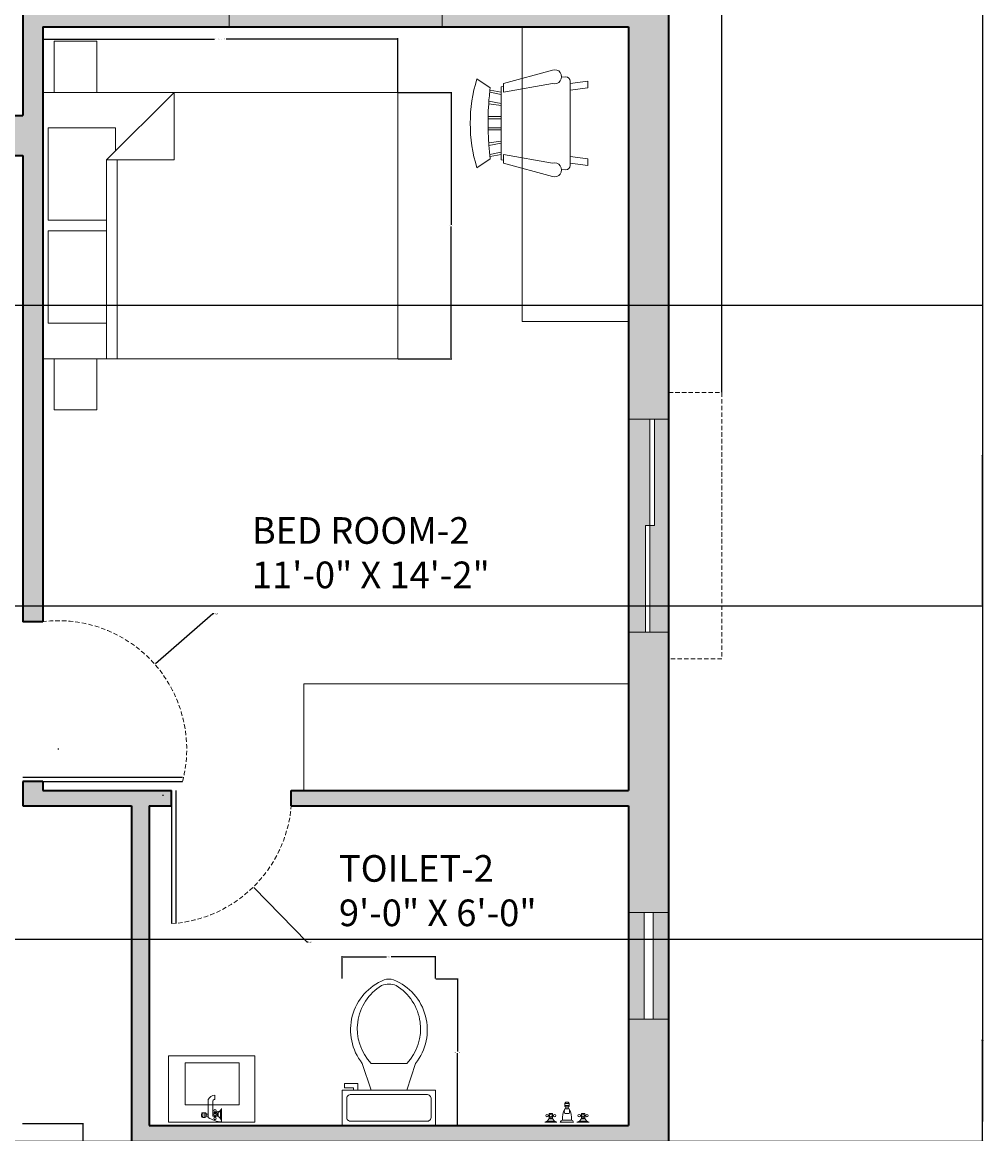
# Model space of a CAD drawing. Units: inches. Extents: x 1693 to 2974, y 2201 to 2965.
# Tile 23 of 24: x 2757 to 2973, y 2588 to 2838. Entities that reach past the tile are written whole.
import ezdxf

# ---------------------------------------------------------------- set-up
doc = ezdxf.new("R2010")
doc.units = ezdxf.units.IN
doc.header["$LTSCALE"] = 2
doc.header["$MEASUREMENT"] = 0
doc.linetypes.add('HIDDEN', pattern=[0.375, 0.25, -0.125])
for name, color, linetype, lineweight in [('A-ANNO-DIMS', 2, 'Continuous', 18), ('A-AREA-IDEN', 7, 'Continuous', 18), ('A-DOOR', 3, 'Continuous', 25), ('A-DOOR-SWNG', 3, 'HIDDEN', 13), ('A-FLOR-CASE', 32, 'Continuous', 18), ('A-FLOR-FIXT', 9, 'Continuous', 18), ('A-FURN', 8, 'Continuous', 18), ('A-GLAZ', 4, 'Continuous', 18), ('A-GLAZ-OVHD', 8, 'HIDDEN', 13), ('A-WALL', 7, 'Continuous', 35)]:
    doc.layers.add(name, color=color, linetype=linetype, lineweight=lineweight)
doc.layers.add('A-GLAZ-PATT', color=141, linetype='Continuous', lineweight=13, true_color=0xadddf7)
doc.layers.add('A-WALL-PATT', color=251, linetype='Continuous', lineweight=13, true_color=0x636466)
doc.styles.get("Standard").update_dxf_attribs({"font": 'arial.ttf'})
doc.dimstyles.get("Standard").update_dxf_attribs({"dimtxt": 0.18, "dimasz": 0.18, "dimexe": 0.18, "dimexo": 0.0625, "dimgap": 0.09, "dimtad": 0, "dimtih": 1, "dimtoh": 1, "dimdec": 1, "dimzin": 0, "dimdsep": 46, "dimlunit": 3, "dimtxsty": 'Standard', "dimcen": 0.09, "dimadec": 0, "dimazin": 0, "dimtfac": 1, "dimtdec": 1, "dimtofl": 0, "dimtmove": 0, "dimatfit": 3, "dimfxl": 1, "dimtolj": 1, "dimtzin": 0, "dimarcsym": 0})

# ---------------------------------------------------------------- blocks, each defined once
blk = doc.blocks.new('Chair - Rocking')
for p, q in [((-8, -4.5), (-10, -1.5)), ((8, -4.5), (10, -1.5)), ((-7.5, -4.5), (-7, -7)), ((-6.5, -7), (-7.02225, -4.43)), ((-4.5, -7), (-4.96674, -4.19951)), ((-4, -7), (-4.40532, -4.16272)), ((-1.5, -4.05012), (-1.5, -7)), ((-1, -7), (-1, -4.05012)), ((1, -7), (1, -4.04655)), ((1.5, -4.05012), (1.5, -7)), ((4, -7), (4.40187, -4.18694)), ((4.5, -7), (4.96761, -4.19437)), ((6.5, -7), (7, -4.4057)), ((7.5, -4.5), (7, -7)), ((-9, -7.5), (-12, -18.49999)), ((-7, -7.5), (-9, -7.5)), ((-9, -18.49999), (-7, -7.5)), ((-8.23428, -6.99939), (-8.3093, -7.47958)), ((-8.23041, -7), (8.23915, -7)), ((7, -7.5), (9, -7.5)), ((9, -18.49999), (7, -7.5)), ((8.31071, -7.48854), (8.23449, -7.00073)), ((9, -7.5), (12, -18.49999)), ((-10.36644, -20.64523), (-10.5, -21.49999)), ((-9, -22.49999), (-9.5, -26.49999)), ((0, -22.49999), (-9.5, -22.49999)), ((-8, -26.49999), (-7.5, -22.49999)), ((0, -22.49999), (9.5, -22.49999)), ((8, -26.49999), (7.5, -22.49999)), ((9, -22.49999), (9.5, -26.49999)), ((10.5, -21.49999), (10.3575, -20.58798)), ((-9.5, -26.49999), (-8, -26.49999)), ((9.5, -26.49999), (8, -26.49999))]:
    blk.add_line(p, q)
for centre, radius, start, end in [((0, -34.08333), 34.08333, 72.93847, 107.0615), ((0, -68.25004), 64.25, 93.92211, 97.15267), ((0, -68.25004), 64.25, 82.84733, 93.92211), ((-10.5, -18.99999), 1.58114, 161.5651, 18.43495), ((10.5, -18.99999), 1.58114, 161.5651, 18.43495), ((-9.5, -21.49999), 1, 180, 270), ((9.5, -21.49999), 1, 270, 0)]:
    blk.add_arc(centre, radius, start, end)
blk = doc.blocks.new('Toilet - top')
for p, q in [((9.5, -6), (9.5, -2)), ((-10, -8.5), (-8, -8.5)), ((-10, -9.5), (-10, -8.5)), ((-7, -9.5), (-10, -9.5)), ((-8, -8.5), (-8, -8)), ((-7, -8), (-7, -9.5)), ((-4, -8), (-6, -14)), ((4, -8), (6, -14)), ((4, -14), (-4, -14))]:
    blk.add_line(p, q)
blk.add_lwpolyline([(10.5, -8), (10.5, 0), (-10.5, 0), (-10.5, -8)], close=True)
for points in [[(-9.5, -2), (-9.5, -6)], [(8.5, -1), (-8.5, -1)], [(-8.5, -7), (8.5, -7)]]:
    blk.add_lwpolyline(points)
for centre, radius, start, end in [((-8.62, -1.88), 0.884, 81.8699, 188.1301), ((8.62, -1.88), 0.884, 351.8699, 98.1301), ((-8.62, -6.12), 0.884, 171.8699, 278.1301), ((8.62, -6.12), 0.884, 261.8699, 8.1301), ((3.52, -21.58), 12.17, 141.4691, 247.9714), ((4.2, -21.82), 11.33, 136.3677, 238.9468), ((-3.52, -21.58), 12.17, 292.0284, 38.5307), ((-4.2, -21.82), 11.33, 301.053, 43.6321), ((0, -27.88), 4, 245.7318, 294.2682), ((0, -29), 4, 254.8605, 285.1395)]:
    blk.add_arc(centre, radius, start, end)
blk = doc.blocks.new('Faucet - Bathroom side')
for p, q in [((-0.625, 4.25), (0.375, 4.25)), ((0.375, 3.75), (-0.625, 3.75)), ((-0.625, 3), (3.375, 3)), ((-0.375, 3), (-0.375, 3.5)), ((0.125, 3.5), (0.125, 3)), ((-1.625, 0), (-1.375, 0)), ((-1.375, 0), (1.375, 0)), ((-0.88366, 0.25), (0.88424, 0.25)), ((-0.375, 1.625), (-0.625, 1.625)), ((-0.375, 1.375), (-0.625, 1.375)), ((0.48078, 0.75), (-0.47286, 0.75)), ((2.875, 2), (0.375, 2)), ((0.375, 1.625), (0.625, 1.625)), ((0.375, 1.375), (0.625, 1.375)), ((4.375, 1.5), (3.375, 1.5))]:
    blk.add_line(p, q)
for points in [[(-0.625, 3.75), (-0.625, 4.25)], [(-0.375, 4.5), (0.125, 4.5)], [(0.125, 3.5), (-0.375, 3.5)], [(0.375, 4.25), (0.375, 3.75)]]:
    blk.add_lwpolyline(points)
blk.add_lwpolyline([(-0.375, 1), (-0.375, 2), (0.375, 2), (0.375, 1)], close=True)
for centre in [(-0.875, 1.5), (0, 1.5), (0.875, 1.5)]:
    blk.add_circle(centre, 0.27951)
for centre, radius, start, end in [((3.45929, -0.0281), 5.08436, 143.4467, 179.6834), ((-0.38253, 4.2575), 0.24259, 88.22243, 181.7776), ((-0.38253, 3.7424), 0.24259, 178.2224, 271.7776), ((0.13252, 4.2575), 0.24259, 358.2224, 91.77757), ((0.13252, 3.7424), 0.24259, 268.2224, 1.777565), ((2.70708, 1.4714), 1.66816, 0.9827695, 66.39737), ((-1.75, 1.375), 1.42522, 285.2551, 344.7449), ((1.75, 1.375), 1.42522, 195.2551, 254.7449), ((-2.49562, -0.286), 3.38273, 9.709485, 29.48735), ((2.96867, 1.5936), 0.41699, 347.0192, 102.9808)]:
    blk.add_arc(centre, radius, start, end)
blk = doc.blocks.new('Faucet - Bathroom front')
for p, q in [((-0.5, 4.25), (0.5, 4.25)), ((0.5, 3.75), (-0.5, 3.75)), ((-0.5, 3), (0.5, 3)), ((-0.25, 3), (-0.25, 3.5)), ((0.25, 3.5), (0.25, 3)), ((-5, 0), (-2.25, 0)), ((-4.5087, 0.25), (-2.7408, 0.25)), ((-4, 1.625), (-4.25, 1.625)), ((-4, 1.375), (-4.25, 1.375)), ((-3.1442, 0.75), (-4.0979, 0.75)), ((-3.25, 1.625), (-3, 1.625)), ((-3.25, 1.375), (-3, 1.375)), ((-1.5, 0), (1.5, 0)), ((-1, 0.5), (1, 0.5)), ((0.5, 2), (-0.5, 2)), ((2.25, 0), (5, 0)), ((2.7413, 0.25), (4.5092, 0.25)), ((3.25, 1.625), (3, 1.625)), ((3.25, 1.375), (3, 1.375)), ((4.1058, 0.75), (3.1521, 0.75)), ((4, 1.625), (4.25, 1.625)), ((4, 1.375), (4.25, 1.375))]:
    blk.add_line(p, q)
for points in [[(-0.5, 3.75), (-0.5, 4.25)], [(-0.25, 4.5), (0.25, 4.5)], [(0.25, 3.5), (-0.25, 3.5)], [(0.5, 4.25), (0.5, 3.75)]]:
    blk.add_lwpolyline(points)
for points in [[(-4, 1), (-4, 2), (-3.25, 2), (-3.25, 1)], [(3.25, 1), (3.25, 2), (4, 2), (4, 1)]]:
    blk.add_lwpolyline(points, close=True)
for centre in [(-4.5, 1.5), (-3.625, 1.5), (-2.75, 1.5), (2.75, 1.5), (3.625, 1.5), (4.5, 1.5)]:
    blk.add_circle(centre, 0.2795)
for centre, radius, start, end in [((3, 1), 4.0311, 150.2551, 187.125), ((0.6413, 2.5), 1.246, 156.3417, 203.6583), ((-0.2575, 4.2575), 0.2426, 88.22243, 181.7776), ((-0.2575, 3.7425), 0.2426, 178.2224, 271.7776), ((0.2575, 4.2575), 0.2426, 358.2224, 91.77757), ((0.2575, 3.7425), 0.2426, 268.2224, 1.777565), ((-3, 1), 4.0311, 352.875, 29.74488), ((-0.6413, 2.5), 1.246, 336.3417, 23.65835), ((-5.375, 1.375), 1.4252, 285.2551, 344.7449), ((-1.875, 1.375), 1.4252, 195.2551, 254.7449), ((-0.7962, -0.2038), 0.7327, 106.1502, 163.8498), ((0.7962, -0.2038), 0.7327, 16.1502, 73.84979), ((1.875, 1.375), 1.4252, 285.2551, 344.7449), ((5.375, 1.375), 1.4252, 195.2551, 254.7449)]:
    blk.add_arc(centre, radius, start, end)
blk = doc.blocks.new('Bed - Queen')
for p, q in [((0, -80.00003), (0, 0)), ((0, 0), (59.99999, 0)), ((59.99999, 0), (59.99999, -80.00003)), ((7.99999, -1.2), (28.79998, -1.2)), ((7.99999, -14.4), (7.99999, -1.2)), ((28.79998, -1.2), (28.79998, -14.4)), ((31.19999, -1.2), (51.99999, -1.2)), ((31.19999, -14.4), (31.19999, -1.2)), ((51.99999, -1.2), (51.99999, -16.4)), ((0, -14.4), (44.8, -14.4)), ((59.99999, -29.6), (44.8, -14.4)), ((44.8, -14.4), (44.8, -29.6)), ((44.8, -16.8), (0, -16.8)), ((51.99999, -16.4), (46.79936, -16.4)), ((44.8, -29.6), (59.99999, -29.6)), ((59.99999, -80.00003), (0, -80.00003))]:
    blk.add_line(p, q)
blk = doc.blocks.new('NIGHTSTAND')
at = {"ltscale": 2}
blk.add_lwpolyline([(11.51, 0), (0, 0), (0, 9.62), (11.51, 9.62)], close=True, dxfattribs=at)
blk = doc.blocks.new('BASIN-WALL-MOUNT')
at = {"ltscale": 2}
for points in [[(15.01, 19.49), (0, 19.49), (0, 0), (15.01, 0)], [(11.1, 15.94), (1.63, 15.94), (1.63, 3.76), (11.1, 3.76)]]:
    blk.add_lwpolyline(points, close=True, dxfattribs=at)
blk = doc.blocks.new('*D37')
at = {"layer": 'A-ANNO-DIMS', "color": 0, "lineweight": -2, "ltscale": 2, "transparency": 16777216}
for p, q in [((2849.8, 2622.8), (2854.87, 2622.8)), ((2854.69, 2622.62), (2854.69, 2606.46)), ((2854.69, 2589.93), (2854.69, 2606.09)), ((2849.8, 2589.75), (2854.87, 2589.75))]:
    blk.add_line(p, q, dxfattribs=at)
at = {"layer": 'A-ANNO-DIMS', "color": 0, "ltscale": 2, "transparency": 16777216}
for points in [[(2854.66, 2622.62), (2854.72, 2622.62), (2854.69, 2622.8)], [(2854.66, 2589.93), (2854.72, 2589.93), (2854.69, 2589.75)]]:
    blk.add_solid(points, dxfattribs=at)
at = {"layer": 'Defpoints', "color": 0, "ltscale": 2, "transparency": 16777216}
for p in [(2849.74, 2622.8), (2849.74, 2589.75), (2854.69, 2589.75)]:
    blk.add_point(p, dxfattribs=at)
at = {"layer": 'A-ANNO-DIMS', "color": 0, "ltscale": 2, "transparency": 16777216, "insert": (2854.69, 2606.28), "char_height": 0.18, "attachment_point": 5}
blk.add_mtext('\\A1;WC 33 TYP.', dxfattribs=at)
blk = doc.blocks.new('*D38')
at = {"layer": 'A-ANNO-DIMS', "color": 0, "lineweight": -2, "ltscale": 2, "transparency": 16777216}
for p, q in [((2828.74, 2622.86), (2828.74, 2627.94)), ((2828.92, 2627.76), (2838.71, 2627.76)), ((2849.56, 2627.76), (2839.77, 2627.76)), ((2849.74, 2622.86), (2849.74, 2627.94))]:
    blk.add_line(p, q, dxfattribs=at)
at = {"layer": 'A-ANNO-DIMS', "color": 0, "ltscale": 2, "transparency": 16777216}
for points in [[(2828.92, 2627.79), (2828.92, 2627.73), (2828.74, 2627.76)], [(2849.56, 2627.79), (2849.56, 2627.73), (2849.74, 2627.76)]]:
    blk.add_solid(points, dxfattribs=at)
at = {"layer": 'Defpoints', "color": 0, "ltscale": 2, "transparency": 16777216}
for p in [(2849.74, 2627.76), (2828.74, 2622.8), (2849.74, 2622.8)]:
    blk.add_point(p, dxfattribs=at)
at = {"layer": 'A-ANNO-DIMS', "color": 0, "ltscale": 2, "transparency": 16777216, "insert": (2839.24, 2627.76), "char_height": 0.18, "attachment_point": 5}
blk.add_mtext('\\A1;21 TYP.', dxfattribs=at)
blk = doc.blocks.new('*D41')
at = {"layer": 'A-ANNO-DIMS', "color": 0, "lineweight": -2, "ltscale": 2, "transparency": 16777216}
for p, q in [((2761.24, 2822.53), (2761.24, 2834.65)), ((2761.42, 2834.47), (2799.93, 2834.47)), ((2841.06, 2834.47), (2802.54, 2834.47)), ((2841.24, 2822.53), (2841.24, 2834.65))]:
    blk.add_line(p, q, dxfattribs=at)
at = {"layer": 'A-ANNO-DIMS', "color": 0, "ltscale": 2, "transparency": 16777216}
for points in [[(2761.42, 2834.5), (2761.42, 2834.44), (2761.24, 2834.47)], [(2841.06, 2834.5), (2841.06, 2834.44), (2841.24, 2834.47)]]:
    blk.add_solid(points, dxfattribs=at)
at = {"layer": 'Defpoints', "color": 0, "ltscale": 2, "transparency": 16777216}
for p in [(2761.24, 2834.47), (2761.24, 2822.47), (2841.24, 2822.47)]:
    blk.add_point(p, dxfattribs=at)
at = {"layer": 'A-ANNO-DIMS', "color": 0, "ltscale": 2, "transparency": 16777216, "insert": (2801.24, 2834.47), "char_height": 0.18, "attachment_point": 5}
blk.add_mtext('\\A1;QUEEN BED 80 TYP.', dxfattribs=at)
blk = doc.blocks.new('*D42')
at = {"layer": 'A-ANNO-DIMS', "color": 0, "lineweight": -2, "ltscale": 2, "transparency": 16777216}
for p, q in [((2841.3, 2822.47), (2853.42, 2822.47)), ((2853.24, 2822.29), (2853.24, 2792.65)), ((2853.24, 2762.65), (2853.24, 2792.29)), ((2841.3, 2762.47), (2853.42, 2762.47))]:
    blk.add_line(p, q, dxfattribs=at)
at = {"layer": 'A-ANNO-DIMS', "color": 0, "ltscale": 2, "transparency": 16777216}
for points in [[(2853.21, 2822.29), (2853.27, 2822.29), (2853.24, 2822.47)], [(2853.21, 2762.65), (2853.27, 2762.65), (2853.24, 2762.47)]]:
    blk.add_solid(points, dxfattribs=at)
at = {"layer": 'Defpoints', "color": 0, "ltscale": 2, "transparency": 16777216}
for p in [(2841.24, 2822.47), (2853.24, 2822.47), (2841.24, 2762.47)]:
    blk.add_point(p, dxfattribs=at)
at = {"layer": 'A-ANNO-DIMS', "color": 0, "ltscale": 2, "transparency": 16777216, "insert": (2853.24, 2792.47), "char_height": 0.18, "attachment_point": 5}
blk.add_mtext('\\A1;60 TYP.', dxfattribs=at)
blk = doc.blocks.new('*D62')
at = {"layer": 'A-ANNO-DIMS', "color": 0, "lineweight": -2, "ltscale": 2, "transparency": 16777216}
for p, q in [((2756.69, 2590.25), (2770.46, 2590.25)), ((2770.28, 2590.07), (2770.28, 2562.93)), ((2770.28, 2535.43), (2770.28, 2562.56)), ((2756.69, 2535.25), (2770.46, 2535.25))]:
    blk.add_line(p, q, dxfattribs=at)
at = {"layer": 'A-ANNO-DIMS', "color": 0, "ltscale": 2, "transparency": 16777216}
for points in [[(2770.25, 2590.07), (2770.31, 2590.07), (2770.28, 2590.25)], [(2770.25, 2535.43), (2770.31, 2535.43), (2770.28, 2535.25)]]:
    blk.add_solid(points, dxfattribs=at)
at = {"layer": 'Defpoints', "color": 0, "ltscale": 2, "transparency": 16777216}
for p in [(2756.63, 2590.25), (2770.28, 2590.25), (2756.63, 2535.25)]:
    blk.add_point(p, dxfattribs=at)
at = {"layer": 'A-ANNO-DIMS', "color": 0, "ltscale": 2, "transparency": 16777216, "insert": (2770.28, 2562.75), "char_height": 0.18, "attachment_point": 5}
blk.add_mtext('\\A1;55 TYP.', dxfattribs=at)
blk = doc.blocks.new('*D81')
at = {"layer": 'A-ANNO-DIMS', "color": 0, "lineweight": -2, "ltscale": 2, "transparency": 16777216}
for p, q in [((1752.34, 2553.91), (1752.34, 2964.96)), ((1752.52, 2964.78), (2332.94, 2964.78)), ((2914.06, 2964.78), (2333.64, 2964.78)), ((2914.24, 2754.97), (2914.24, 2964.96))]:
    blk.add_line(p, q, dxfattribs=at)
at = {"layer": 'A-ANNO-DIMS', "color": 0, "ltscale": 2, "transparency": 16777216}
for points in [[(1752.52, 2964.81), (1752.52, 2964.75), (1752.34, 2964.78)], [(2914.06, 2964.81), (2914.06, 2964.75), (2914.24, 2964.78)]]:
    blk.add_solid(points, dxfattribs=at)
at = {"layer": 'Defpoints', "color": 0, "ltscale": 2, "transparency": 16777216}
for p in [(2914.24, 2964.78), (2914.24, 2754.9), (1752.34, 2553.84)]:
    blk.add_point(p, dxfattribs=at)
at = {"layer": 'A-ANNO-DIMS', "color": 0, "ltscale": 2, "transparency": 16777216, "insert": (2333.29, 2964.78), "char_height": 0.18, "attachment_point": 5}
blk.add_mtext('\\A1;1162', dxfattribs=at)
blk = doc.blocks.new('*D87')
at = {"layer": 'A-ANNO-DIMS', "color": 0, "lineweight": -2, "ltscale": 2, "transparency": 16777216}
for p, q in [((2902.3, 2846.25), (2973.12, 2846.25)), ((2972.94, 2846.07), (2972.94, 2590.69)), ((2972.94, 2334.93), (2972.94, 2590.32)), ((2902.3, 2334.75), (2973.12, 2334.75))]:
    blk.add_line(p, q, dxfattribs=at)
at = {"layer": 'A-ANNO-DIMS', "color": 0, "ltscale": 2, "transparency": 16777216}
for points in [[(2972.91, 2846.07), (2972.97, 2846.07), (2972.94, 2846.25)], [(2972.91, 2334.93), (2972.97, 2334.93), (2972.94, 2334.75)]]:
    blk.add_solid(points, dxfattribs=at)
at = {"layer": 'Defpoints', "color": 0, "ltscale": 2, "transparency": 16777216}
for p in [(2902.24, 2846.25), (2972.94, 2846.25), (2902.24, 2334.75)]:
    blk.add_point(p, dxfattribs=at)
at = {"layer": 'A-ANNO-DIMS', "color": 0, "ltscale": 2, "transparency": 16777216, "insert": (2972.94, 2590.5), "char_height": 0.18, "attachment_point": 5}
blk.add_mtext('\\A1;511.5', dxfattribs=at)
blk = doc.blocks.new('*D90')
at = {"layer": 'A-ANNO-DIMS', "color": 0, "lineweight": -2, "ltscale": 2, "transparency": 16777216}
for p, q in [((2145.8, 2774.54), (2973.12, 2774.54)), ((2972.94, 2774.36), (2972.94, 2740.87)), ((2972.94, 2707.02), (2972.94, 2740.51)), ((2294.3, 2706.84), (2973.12, 2706.84))]:
    blk.add_line(p, q, dxfattribs=at)
at = {"layer": 'A-ANNO-DIMS', "color": 0, "ltscale": 2, "transparency": 16777216}
for points in [[(2972.91, 2774.36), (2972.97, 2774.36), (2972.94, 2774.54)], [(2972.91, 2707.02), (2972.97, 2707.02), (2972.94, 2706.84)]]:
    blk.add_solid(points, dxfattribs=at)
at = {"layer": 'Defpoints', "color": 0, "ltscale": 2, "transparency": 16777216}
for p in [(2145.74, 2774.54), (2294.24, 2706.84), (2972.94, 2706.84)]:
    blk.add_point(p, dxfattribs=at)
at = {"layer": 'A-ANNO-DIMS', "color": 0, "ltscale": 2, "transparency": 16777216, "insert": (2972.94, 2740.69), "char_height": 0.18, "attachment_point": 5}
blk.add_mtext('\\A1;67.7', dxfattribs=at)
blk = doc.blocks.new('*D97')
at = {"layer": 'A-ANNO-DIMS', "color": 0, "lineweight": -2, "ltscale": 2, "transparency": 16777216}
for p, q in [((2294.3, 2631.75), (2973.12, 2631.75)), ((2972.94, 2631.57), (2972.94, 2609.19)), ((2972.94, 2586.44), (2972.94, 2608.83)), ((2294.3, 2586.26), (2973.12, 2586.26))]:
    blk.add_line(p, q, dxfattribs=at)
at = {"layer": 'A-ANNO-DIMS', "color": 0, "ltscale": 2, "transparency": 16777216}
for points in [[(2972.91, 2631.57), (2972.97, 2631.57), (2972.94, 2631.75)], [(2972.91, 2586.44), (2972.97, 2586.44), (2972.94, 2586.26)]]:
    blk.add_solid(points, dxfattribs=at)
at = {"layer": 'Defpoints', "color": 0, "ltscale": 2, "transparency": 16777216}
for p in [(2294.24, 2631.75), (2972.94, 2631.75), (2294.24, 2586.26)]:
    blk.add_point(p, dxfattribs=at)
at = {"layer": 'A-ANNO-DIMS', "color": 0, "ltscale": 2, "transparency": 16777216, "insert": (2972.94, 2609.01), "char_height": 0.18, "attachment_point": 5}
blk.add_mtext('\\A1;45.49', dxfattribs=at)
blk = doc.blocks.new('*D122')
at = {"layer": 'A-ANNO-DIMS', "color": 0, "lineweight": -2, "ltscale": 2, "transparency": 16777216}
for p, q in [((2788.28, 2664.16), (2788.46, 2664.16)), ((2788.37, 2664.07), (2788.37, 2664.25)), ((2820.83, 2631.09), (2808.79, 2643.36)), ((2821.01, 2631.09), (2820.83, 2631.09))]:
    blk.add_line(p, q, dxfattribs=at)
at = {"layer": 'A-ANNO-DIMS', "color": 0, "ltscale": 2, "transparency": 16777216}
blk.add_solid([(2808.81, 2643.38), (2808.77, 2643.34), (2808.66, 2643.49)], dxfattribs=at)
at = {"layer": 'Defpoints', "color": 0, "ltscale": 2, "transparency": 16777216}
for p in [(2788.37, 2664.16), (2808.66, 2643.49)]:
    blk.add_point(p, dxfattribs=at)
at = {"layer": 'A-ANNO-DIMS', "color": 0, "ltscale": 2, "transparency": 16777216, "insert": (2821.49, 2631.09), "char_height": 0.18, "attachment_point": 5}
blk.add_mtext('\\A1;R28.96', dxfattribs=at)
blk = doc.blocks.new('*D123')
at = {"layer": 'A-ANNO-DIMS', "color": 0, "lineweight": -2, "ltscale": 2, "transparency": 16777216}
for p, q in [((2799.58, 2705.02), (2786.67, 2693.73)), ((2799.76, 2705.02), (2799.58, 2705.02)), ((2764.71, 2674.59), (2764.89, 2674.59)), ((2764.8, 2674.5), (2764.8, 2674.68))]:
    blk.add_line(p, q, dxfattribs=at)
at = {"layer": 'A-ANNO-DIMS', "color": 0, "ltscale": 2, "transparency": 16777216}
blk.add_solid([(2786.65, 2693.75), (2786.69, 2693.71), (2786.54, 2693.61)], dxfattribs=at)
at = {"layer": 'Defpoints', "color": 0, "ltscale": 2, "transparency": 16777216}
for p in [(2786.54, 2693.61), (2764.8, 2674.59)]:
    blk.add_point(p, dxfattribs=at)
at = {"layer": 'A-ANNO-DIMS', "color": 0, "ltscale": 2, "transparency": 16777216, "insert": (2800.31, 2705.02), "char_height": 0.18, "attachment_point": 5}
blk.add_mtext('\\A1;R28.887', dxfattribs=at)

msp = doc.modelspace()

# ---------------------------------------------------------------- hatches: boundary and pattern name
at = {"layer": 'A-GLAZ-PATT', "ltscale": 2}
h = msp.add_hatch(color=256, dxfattribs=at)
h.dxf.hatch_style = 1
h.paths.add_polyline_path([(2656.9702, 2338.2547), (2632.9702, 2338.2547), (2632.9702, 2339.2547), (2608.9702, 2339.2547), (2608.9702, 2334.7547), (2656.9702, 2334.7547)])
h.paths.add_polyline_path([(2656.9702, 2343.7547), (2608.9702, 2343.7547), (2608.9702, 2340.2547), (2632.9702, 2340.2547), (2632.9702, 2339.2547), (2656.9702, 2339.2547)])
h.paths.add_polyline_path([(2775.7544, 2338.2547), (2751.7544, 2338.2547), (2751.7544, 2334.7547), (2775.7544, 2334.7547)])
h.paths.add_polyline_path([(2775.7544, 2343.7547), (2751.7544, 2343.7547), (2751.7544, 2340.2547), (2775.7544, 2340.2547)])
h.paths.add_polyline_path([(2897.7363, 2568.7999), (2893.2363, 2568.7999), (2893.2363, 2520.7999), (2896.7363, 2520.7999), (2896.7363, 2544.7999), (2897.7363, 2544.7999)])
h.paths.add_polyline_path([(2902.2363, 2568.7999), (2898.7363, 2568.7999), (2898.7363, 2544.7999), (2897.7363, 2544.7999), (2897.7363, 2520.7999), (2902.2363, 2520.7999)])
h.paths.add_polyline_path([(2902.2363, 2637.7547), (2898.7363, 2637.7547), (2898.7363, 2613.7547), (2902.2363, 2613.7547)])
h.paths.add_polyline_path([(2896.7363, 2637.7547), (2893.2363, 2637.7547), (2893.2363, 2613.7547), (2896.7363, 2613.7547)])
h.paths.add_polyline_path([(2902.2363, 2748.903), (2899.0477, 2748.903), (2899.0477, 2724.903), (2898.0477, 2724.903), (2898.0477, 2700.903), (2902.2363, 2700.903)])
h.paths.add_polyline_path([(2898.0477, 2748.903), (2893.2363, 2748.903), (2893.2363, 2700.903), (2897.0477, 2700.903), (2897.0477, 2724.903), (2898.0477, 2724.903)])
h.paths.add_polyline_path([(2851.2363, 2846.2547), (2803.2363, 2846.2547), (2803.2363, 2842.7547), (2827.2363, 2842.7547), (2827.2363, 2841.7547), (2851.2363, 2841.7547)])
h.paths.add_polyline_path([(2851.2363, 2840.7547), (2827.2363, 2840.7547), (2827.2363, 2841.7547), (2803.2363, 2841.7547), (2803.2363, 2837.2547), (2851.2363, 2837.2547)])
h.paths.add_polyline_path([(2578.2363, 2846.2547), (2530.2363, 2846.2547), (2530.2363, 2842.7547), (2554.2363, 2842.7547), (2554.2363, 2841.7547), (2578.2363, 2841.7547)])
h.paths.add_polyline_path([(2578.2363, 2840.7547), (2554.2363, 2840.7547), (2554.2363, 2841.7547), (2530.2363, 2841.7547), (2530.2363, 2837.2547), (2578.2363, 2837.2547)])
h.paths.add_polyline_path([(2732.7363, 2812.7547), (2705.1363, 2812.7547), (2705.1363, 2811.7547), (2676.3363, 2811.7547), (2676.3363, 2812.7547), (2648.7363, 2812.7547), (2648.7363, 2808.2547), (2732.7363, 2808.2547)])
h.paths.add_polyline_path([(2732.7363, 2817.2547), (2648.7363, 2817.2547), (2648.7363, 2813.7547), (2676.3363, 2813.7547), (2676.3363, 2812.7547), (2705.1363, 2812.7547), (2705.1363, 2813.7547), (2732.7363, 2813.7547)])
h.paths.add_polyline_path([(2488.2363, 2695.8203), (2484.7878, 2695.8203), (2484.7878, 2671.8203), (2488.2363, 2671.8203)])
h.paths.add_polyline_path([(2482.7878, 2695.8203), (2479.2363, 2695.8203), (2479.2363, 2671.8203), (2482.7878, 2671.8203)])
h.paths.add_polyline_path([(2488.2363, 2572.4371), (2484.7363, 2572.4371), (2484.7363, 2541.4371), (2483.7363, 2541.4371), (2483.7363, 2512.4371), (2488.2363, 2512.4371)])
h.paths.add_polyline_path([(2482.7363, 2541.4371), (2483.7363, 2541.4371), (2483.7363, 2572.4371), (2479.2363, 2572.4371), (2479.2363, 2512.4371), (2482.7363, 2512.4371)])
h.paths.add_polyline_path([(2248.9863, 2706.8449), (2190.9863, 2706.8449), (2190.9863, 2703.3449), (2219.9863, 2703.3449), (2219.9863, 2702.3449), (2248.9863, 2702.3449)])
h.paths.add_polyline_path([(2248.9863, 2701.3449), (2219.9863, 2701.3449), (2219.9863, 2702.3449), (2190.9863, 2702.3449), (2190.9863, 2697.8449), (2248.9863, 2697.8449)])
h.paths.add_polyline_path([(2151.9207, 2293.3449), (2127.9207, 2293.3449), (2127.9207, 2289.8449), (2151.9207, 2289.8449)])
h.paths.add_polyline_path([(2151.9207, 2298.8449), (2127.9207, 2298.8449), (2127.9207, 2295.3449), (2151.9207, 2295.3449)])
h.paths.add_polyline_path([(2084.023, 2293.3449), (2066.023, 2293.3449), (2066.023, 2294.3449), (2048.023, 2294.3449), (2048.023, 2289.8449), (2084.023, 2289.8449)])
h.paths.add_polyline_path([(2084.023, 2298.8449), (2048.023, 2298.8449), (2048.023, 2295.3449), (2066.023, 2295.3449), (2066.023, 2294.3449), (2084.023, 2294.3449)])
h.paths.add_polyline_path([(1966.0781, 2293.3449), (1948.0781, 2293.3449), (1948.0781, 2294.3449), (1930.0781, 2294.3449), (1930.0781, 2289.8449), (1966.0781, 2289.8449)])
h.paths.add_polyline_path([(1966.0781, 2298.8449), (1930.0781, 2298.8449), (1930.0781, 2295.3449), (1948.0781, 2295.3449), (1948.0781, 2294.3449), (1966.0781, 2294.3449)])
h.paths.add_polyline_path([(1787.2363, 2403.1922), (1782.7363, 2403.1922), (1782.7363, 2355.1922), (1786.2363, 2355.1922), (1786.2363, 2379.1922), (1787.2363, 2379.1922)])
h.paths.add_polyline_path([(1791.7363, 2403.1922), (1788.2363, 2403.1922), (1788.2363, 2379.1922), (1787.2363, 2379.1922), (1787.2363, 2355.1922), (1791.7363, 2355.1922)])
h.paths.add_polyline_path([(1786.2363, 2477.5455), (1782.7363, 2477.5455), (1782.7363, 2453.5455), (1786.2363, 2453.5455)])
h.paths.add_polyline_path([(1791.7363, 2477.5455), (1788.2363, 2477.5455), (1788.2363, 2453.5455), (1791.7363, 2453.5455)])
h.paths.add_polyline_path([(1786.2363, 2621.6433), (1782.7363, 2621.6433), (1782.7363, 2585.6433), (1786.2363, 2585.6433)])
h.paths.add_polyline_path([(1791.7363, 2621.6433), (1788.2363, 2621.6433), (1788.2363, 2585.6433), (1791.7363, 2585.6433)])
h.paths.add_polyline_path([(1908.1286, 2706.8449), (1860.1286, 2706.8449), (1860.1286, 2703.3449), (1884.1286, 2703.3449), (1884.1286, 2702.3449), (1908.1286, 2702.3449)])
h.paths.add_polyline_path([(1908.1286, 2701.3449), (1884.1286, 2701.3449), (1884.1286, 2702.3449), (1860.1286, 2702.3449), (1860.1286, 2697.8449), (1908.1286, 2697.8449)])
h.paths.add_polyline_path([(1973.9863, 2706.8449), (1949.9863, 2706.8449), (1949.9863, 2703.3449), (1973.9863, 2703.3449)])
h.paths.add_polyline_path([(1973.9863, 2701.3449), (1949.9863, 2701.3449), (1949.9863, 2697.8449), (1973.9863, 2697.8449)])
h.paths.add_polyline_path([(2112.7363, 2690.3449), (2028.7363, 2690.3449), (2028.7363, 2686.8449), (2056.3363, 2686.8449), (2056.3363, 2685.8449), (2085.1363, 2685.8449), (2085.1363, 2686.8449), (2112.7363, 2686.8449)])
h.paths.add_polyline_path([(2112.7363, 2685.8449), (2085.1363, 2685.8449), (2085.1363, 2684.8449), (2056.3363, 2684.8449), (2056.3363, 2685.8449), (2028.7363, 2685.8449), (2028.7363, 2681.3449), (2112.7363, 2681.3449)])
h.paths.add_polyline_path([(2422.7363, 2640.7547), (2350.7363, 2640.7547), (2350.7363, 2637.2547), (2386.7363, 2637.2547), (2386.7363, 2636.2547), (2422.7363, 2636.2547)])
h.paths.add_polyline_path([(2422.7363, 2635.2547), (2386.7363, 2635.2547), (2386.7363, 2636.2547), (2350.7363, 2636.2547), (2350.7363, 2631.7547), (2422.7363, 2631.7547)])
at = {"layer": 'A-WALL-PATT', "ltscale": 2}
h = msp.add_hatch(color=256, dxfattribs=at)
h.dxf.hatch_style = 1
h.paths.add_polyline_path([(1928.2363, 2733.2161), (1930.9384, 2733.2161), (1930.9384, 2737.2161), (1923.7363, 2737.2161), (1923.7363, 2706.8449), (1908.1286, 2706.8449), (1908.1286, 2697.8449), (1923.7363, 2697.8449), (1923.7363, 2692.8449), (1928.2363, 2692.8449), (1928.2363, 2697.8449), (1949.9863, 2697.8449), (1949.9863, 2706.8449), (1928.2363, 2706.8449)])
h.paths.add_polyline_path([(2004.7363, 2737.2161), (1995.7363, 2737.2161), (1995.7363, 2706.8449), (1985.6374, 2706.8449), (1973.9863, 2706.8449), (1973.9863, 2697.8449), (2000.2363, 2697.8449), (2000.2363, 2686.5348), (2000.3613, 2686.5348), (2000.3613, 2667.0432), (2000.2363, 2601.8449), (1928.2363, 2601.8449), (1928.2363, 2662.8449), (1923.7363, 2662.8449), (1923.7363, 2595.3449), (1928.2363, 2595.3449), (1928.2363, 2597.3449), (2004.7363, 2597.3449), (2004.7363, 2681.3449), (2012.7814, 2681.3449), (2028.7363, 2681.3449), (2028.7363, 2690.3449), (2004.7363, 2690.3449)])
h.paths.add_polyline_path([(2190.9863, 2706.8449), (2184.9863, 2706.8449), (2145.7363, 2706.8449), (2145.7363, 2765.3449), (2145.7363, 2774.5394), (2136.7363, 2774.5394), (2136.7363, 2756.3449), (2136.7363, 2690.3449), (2112.7363, 2690.3449), (2112.7363, 2681.3449), (2136.7363, 2681.3449), (2136.7363, 2597.3449), (2141.2363, 2597.3449), (2141.2363, 2697.8449), (2190.9863, 2697.8449)])
h.paths.add_polyline_path([(1860.1286, 2706.8449), (1782.7363, 2706.8449), (1782.7363, 2621.6433), (1791.7363, 2621.6433), (1791.7363, 2697.8449), (1860.1286, 2697.8449)])
h.paths.add_polyline_path([(1791.7363, 2585.6433), (1782.7363, 2585.6433), (1782.7363, 2562.8449), (1782.7363, 2553.8449), (1752.3363, 2553.8449), (1752.3363, 2544.2586), (1756.3363, 2544.2586), (1756.3363, 2549.3449), (1782.7363, 2549.3449), (1782.7363, 2489.2404), (1782.7363, 2477.5455), (1791.7363, 2477.5455), (1791.7363, 2493.5991), (1791.6113, 2493.5991), (1791.6113, 2513.0907), (1791.6824, 2533.7198, -0.94742783), (1791.7363, 2534.7168), (1791.7363, 2549.3449), (1863.7363, 2549.3449), (1863.7363, 2513.3449), (1866.7363, 2513.3449), (1866.7363, 2549.3449), (1924.7363, 2549.3449), (1924.7363, 2447.3449), (1924.7363, 2442.8449), (1933.7363, 2442.8449), (1933.7363, 2447.3449), (1928.2363, 2447.3449), (1928.2363, 2559.3449), (1923.7363, 2559.3449), (1923.7363, 2553.8449), (1791.7363, 2553.8449), (1791.7363, 2562.8449)])
h.paths.add_polyline_path([(1791.7363, 2442.8449), (1866.7363, 2442.8449), (1866.7363, 2447.3449), (1866.7363, 2483.3449), (1863.7363, 2483.3449), (1863.7363, 2447.3449), (1791.7363, 2447.3449), (1791.7363, 2453.5455), (1782.7363, 2453.5455), (1782.7363, 2447.3449), (1756.3363, 2447.3449), (1756.3363, 2455.7126), (1752.3363, 2455.7126), (1752.3363, 2442.8449), (1782.7363, 2442.8449), (1782.7363, 2403.1922), (1791.7363, 2403.1922)])
h.paths.add_polyline_path([(1930.0781, 2298.8449), (1791.7363, 2298.8449), (1791.7363, 2355.1922), (1782.7363, 2355.1922), (1782.7363, 2289.8449), (1930.0781, 2289.8449)])
h.paths.add_polyline_path([(2624.7363, 2883.2547), (2624.7363, 2902.6165), (2624.7363, 2906.0761), (2615.7363, 2906.0761), (2615.7363, 2892.2547), (2615.7363, 2846.2547), (2578.2363, 2846.2547), (2578.2363, 2837.2547), (2620.2363, 2837.2547), (2620.2363, 2743.2547), (2624.7363, 2743.2547), (2624.7363, 2808.2547), (2648.7363, 2808.2547), (2648.7363, 2817.2547), (2624.7363, 2817.2547)])
h.paths.add_polyline_path([(2530.2363, 2846.2547), (2479.2363, 2846.2547), (2479.2363, 2695.8203), (2488.2363, 2695.8203), (2488.2363, 2700.7547), (2567.2363, 2700.7547), (2567.2363, 2705.2547), (2488.2363, 2705.2547), (2488.2363, 2837.2547), (2530.2363, 2837.2547)])
h.paths.add_polyline_path([(2488.2363, 2487.7547), (2630.2363, 2487.7547, -0.00990191), (2630.2363, 2489.0322), (2630.2363, 2492.2547), (2488.2363, 2492.2547), (2488.2363, 2512.4371), (2479.2363, 2512.4371), (2479.2363, 2334.7547), (2608.9702, 2334.7547), (2608.9702, 2343.7547), (2488.2363, 2343.7547)])
h.paths.add_polyline_path([(2751.7544, 2343.7547), (2672.7363, 2343.7547), (2672.7363, 2409.7547), (2674.7363, 2409.7547), (2674.7363, 2413.7547), (2672.7363, 2413.7547), (2672.7363, 2487.7547), (2732.7363, 2487.7547), (2732.7363, 2413.7547), (2704.7363, 2413.7547), (2704.7363, 2409.7547), (2784.7363, 2409.7547), (2784.7363, 2343.7547), (2775.7544, 2343.7547), (2775.7544, 2334.7547), (2902.2363, 2334.7547), (2902.2363, 2520.7999), (2893.2363, 2520.7999), (2893.2363, 2413.7547), (2856.0145, 2413.7547), (2856.0145, 2409.7547), (2893.2363, 2409.7547), (2893.2363, 2343.7547), (2789.2363, 2343.7547), (2789.2363, 2409.7547), (2819.2363, 2409.7547), (2826.0145, 2409.7547), (2826.0145, 2413.7547), (2789.2363, 2413.7547), (2789.2363, 2492.2547), (2784.7363, 2492.2547), (2784.7363, 2413.7547), (2736.7363, 2413.7547), (2736.7363, 2492.2547), (2672.7363, 2492.2547), (2666.2363, 2492.2547), (2666.2363, 2487.7547), (2668.2363, 2487.7547), (2668.2363, 2343.7547), (2656.9702, 2343.7547), (2656.9702, 2334.7547), (2662.9702, 2334.7547), (2751.7544, 2334.7547)])
h.paths.add_polyline_path([(2902.2363, 2613.7547), (2893.2363, 2613.7547), (2893.2363, 2589.7547), (2785.2363, 2589.7547), (2785.2363, 2661.7547), (2790.2363, 2661.7547), (2790.2363, 2665.2547), (2761.2363, 2665.2547), (2761.2363, 2667.2547), (2756.7363, 2667.2547), (2756.7363, 2661.7547), (2781.2363, 2661.7547), (2781.2363, 2585.7547), (2893.2363, 2585.7547), (2893.2363, 2568.7999), (2902.2363, 2568.7999)])
h.paths.add_polyline_path([(2488.2363, 2671.8203), (2479.2363, 2671.8203), (2479.2363, 2645.2547), (2479.2363, 2623.4598), (2488.2363, 2623.4598), (2488.2363, 2636.2547), (2624.7363, 2636.2547), (2624.7363, 2640.7547), (2603.7363, 2640.7547), (2603.7363, 2700.7547), (2624.7363, 2700.7547), (2624.7363, 2707.2547), (2620.2363, 2707.2547), (2620.2363, 2705.2547), (2597.2363, 2705.2547), (2597.2363, 2700.7547), (2599.2363, 2700.7547), (2599.2363, 2640.7547), (2488.2363, 2640.7547)])
h.paths.add_polyline_path([(2761.2363, 2837.2547), (2803.2363, 2837.2547), (2803.2363, 2846.2547), (2797.2363, 2846.2547), (2765.7363, 2846.2547), (2756.7363, 2846.2547), (2756.7363, 2817.2547), (2732.7363, 2817.2547), (2732.7363, 2808.2547), (2756.7363, 2808.2547), (2756.7363, 2703.2547), (2761.2363, 2703.2547)])
h.paths.add_polyline_path([(2739.7489, 2433.1234), (2786.9181, 2433.1234), (2786.9181, 2455.5122), (2739.7489, 2455.5122)], flags=25)
h = msp.add_hatch(color=256, dxfattribs=at)
h.dxf.hatch_style = 1
h.paths.add_polyline_path([(2902.2363, 2846.2547), (2851.2363, 2846.2547), (2851.2363, 2837.2547), (2893.2363, 2837.2547), (2893.2363, 2748.903), (2902.2363, 2748.903), (2902.2363, 2754.903)])
h.paths.add_polyline_path([(2902.2363, 2700.903), (2893.2363, 2700.903), (2893.2363, 2665.2547), (2817.2363, 2665.2547), (2817.2363, 2661.7547), (2893.2363, 2661.7547), (2893.2363, 2637.7547), (2902.2363, 2637.7547)])

# ---------------------------------------------------------------- linework, layer by layer
at = {"layer": 'A-DOOR', "ltscale": 2}
for p, q in [((2756.7363, 2668.2547), (2792.7363, 2668.2547)), ((2756.7363, 2667.2547), (2792.7363, 2667.2547)), ((2790.2363, 2665.2547), (2790.2363, 2635.2547)), ((2791.2363, 2665.2547), (2791.2363, 2635.2547))]:
    msp.add_line(p, q, dxfattribs=at)
at = {"layer": 'A-DOOR-SWNG', "ltscale": 2}
for centre, radius, start, end in [((2764.7956, 2674.5879), 28.8869, 345.294094, 97.077756), ((2788.3744, 2664.1565), 28.9617, 273.686051, 355.243031)]:
    msp.add_arc(centre, radius, start, end, dxfattribs=at)
at = {"layer": 'A-FLOR-CASE'}
msp.add_line((2869.2363, 2837.2547), (2869.2363, 2770.8328), dxfattribs=at)
at = {"layer": 'A-FLOR-CASE', "ltscale": 2}
for p, q in [((2893.2363, 2770.8328), (2869.2363, 2770.8328)), ((2820.093, 2689.2547), (2893.2363, 2689.2547)), ((2820.093, 2689.2547), (2820.093, 2665.2547))]:
    msp.add_line(p, q, dxfattribs=at)
at = {"layer": 'A-GLAZ', "ltscale": 2}
for p, q in [((2803.2363, 2837.2547), (2803.2363, 2846.2547)), ((2851.2363, 2837.2547), (2851.2363, 2846.2547)), ((2893.2363, 2748.903), (2902.2363, 2748.903)), ((2898.0477, 2748.903), (2898.0477, 2700.903)), ((2899.0477, 2748.903), (2899.0477, 2724.903)), ((2897.0477, 2724.903), (2897.0477, 2700.903)), ((2897.0477, 2724.903), (2899.0477, 2724.903)), ((2899.0477, 2724.903), (2897.0477, 2724.903)), ((2893.2363, 2700.903), (2902.2363, 2700.903)), ((2893.2363, 2637.7547), (2902.2363, 2637.7547)), ((2896.7363, 2637.7547), (2896.7363, 2613.7547)), ((2898.7363, 2637.7547), (2898.7363, 2613.7547)), ((2893.2363, 2613.7547), (2902.2363, 2613.7547))]:
    msp.add_line(p, q, dxfattribs=at)
at = {"layer": 'A-GLAZ-OVHD', "ltscale": 2}
for p, q in [((2902.2363, 2748.903), (2902.2363, 2754.903)), ((2902.2363, 2754.903), (2914.2363, 2754.903)), ((2914.2363, 2754.903), (2914.2363, 2700.903)), ((2914.2363, 2700.903), (2914.2363, 2694.903)), ((2914.2363, 2694.903), (2902.2363, 2694.903))]:
    msp.add_line(p, q, dxfattribs=at)
at = {"layer": 'A-WALL'}
for p, q in [((2756.7363, 2877.2547), (2756.7363, 2817.2547)), ((2902.2363, 2846.2547), (2902.2363, 2334.7547)), ((2761.2363, 2837.2547), (2761.2363, 2703.2547)), ((2893.2363, 2837.2547), (2893.2363, 2665.2547)), ((2756.7363, 2808.2547), (2756.7363, 2703.2547)), ((2756.7363, 2667.2547), (2756.7363, 2661.7547)), ((2761.2363, 2667.2547), (2761.2363, 2665.2547)), ((2781.2363, 2661.7547), (2781.2363, 2585.7547)), ((2785.2363, 2661.7547), (2785.2363, 2589.7547)), ((2893.2363, 2661.7547), (2893.2363, 2589.7547))]:
    msp.add_line(p, q, dxfattribs=at)
at = {"layer": 'A-WALL', "ltscale": 2}
for p, q in [((2761.2363, 2837.2547), (2893.2363, 2837.2547)), ((2624.7363, 2817.2547), (2756.7363, 2817.2547)), ((2624.7363, 2808.2547), (2756.7363, 2808.2547)), ((2761.2363, 2703.2547), (2756.7363, 2703.2547)), ((2761.2363, 2667.2547), (2756.7363, 2667.2547)), ((2761.2363, 2665.2547), (2790.2363, 2665.2547)), ((2790.2363, 2661.7547), (2790.2363, 2665.2547)), ((2817.2363, 2661.7547), (2817.2363, 2665.2547)), ((2817.2363, 2665.2547), (2893.2363, 2665.2547)), ((2756.7363, 2661.7547), (2781.2363, 2661.7547)), ((2785.2363, 2661.7547), (2790.2363, 2661.7547)), ((2817.2363, 2661.7547), (2893.2363, 2661.7547)), ((2785.2363, 2589.7547), (2893.2363, 2589.7547))]:
    msp.add_line(p, q, dxfattribs=at)

# ---------------------------------------------------------------- block references
at = {"layer": 'A-FLOR-FIXT', "ltscale": 2, "xscale": -1, "rotation": 180}
msp.add_blockref('Toilet - top', (2839.2363, 2589.7547), dxfattribs=at)
at = {"layer": 'A-FLOR-FIXT', "rotation": 270.0000000000048}
msp.add_blockref('BASIN-WALL-MOUNT', (2789.565, 2605.5136), dxfattribs=at)
at = {"layer": 'A-FLOR-FIXT', "ltscale": 2, "rotation": 89.99999999999996}
msp.add_blockref('Faucet - Bathroom side', (2801.5459, 2592.2503), dxfattribs=at)
at = {"layer": 'A-FLOR-FIXT', "ltscale": 2}
msp.add_blockref('Faucet - Bathroom front', (2879.3418, 2590.5067), dxfattribs=at)
at = {"layer": 'A-FURN', "rotation": 270.0000000000031}
for p in [(2763.8504, 2833.9797), (2763.8504, 2762.4699)]:
    msp.add_blockref('NIGHTSTAND', p, dxfattribs=at)
at = {"layer": 'A-FURN', "ltscale": 2, "xscale": -1, "rotation": 90}
msp.add_blockref('Chair - Rocking', (2857.5571, 2815.4991), dxfattribs=at)
at = {"layer": 'A-FURN', "ltscale": 2, "rotation": 89.99999999999999}
msp.add_blockref('Bed - Queen', (2761.2363, 2762.4698), dxfattribs=at)

# ---------------------------------------------------------------- texts
at = {"layer": 'A-AREA-IDEN', "ltscale": 2, "char_height": 6, "attachment_point": 1}
for s, insert in [('BED ROOM-2\\P11\'-0" X 14\'-2"', (2808.3553, 2726.7983)), ('TOILET-2\\P9\'-0" X 6\'-0"', (2827.9712, 2650.6843))]:
    msp.add_mtext_dynamic_manual_height_columns(s, width=108.452746, gutter_width=1, heights=[0], dxfattribs=dict(at, insert=insert))

# ---------------------------------------------------------------- dimensions: what is measured, and where the dimension line sits
at = {"layer": 'A-ANNO-DIMS', "ltscale": 2}
dim = msp.add_linear_dim(base=(2914.2363, 2964.7761), p1=(1752.3363, 2553.8449), p2=(2914.2363, 2754.903), dimstyle='Standard', override={"dimdec": 0, "dimlfac": 1, "dimrnd": 0, "dimzin": 0, "dimdsep": 46, "dimlunit": 2}, dxfattribs=at)
dim.commit()
dim.dimension.update_dxf_attribs({"geometry": '*D81', "text_midpoint": (2333.2863, 2964.7761)})
for base, p1, p2, override, picture, middle in [((2972.9363, 2846.2547), (2902.2363, 2334.7547), (2902.2363, 2846.2547), {"dimdec": 1, "dimlfac": 1, "dimrnd": 0, "dimzin": 0, "dimdsep": 46, "dimlunit": 2}, '*D87', (2972.9363, 2590.5047)), ((2972.9363, 2706.8449), (2145.7363, 2774.5394), (2294.2363, 2706.8449), {"dimdec": 1, "dimlfac": 1, "dimrnd": 0, "dimzin": 0, "dimdsep": 46, "dimlunit": 2}, '*D90', (2972.9363, 2740.6922)), ((2972.9363, 2631.7547), (2294.2363, 2586.2648), (2294.2363, 2631.7547), {"dimdec": 2, "dimlfac": 1, "dimrnd": 0, "dimzin": 0, "dimdsep": 46, "dimlunit": 2}, '*D97', (2972.9363, 2609.0097))]:
    dim = msp.add_linear_dim(base=base, p1=p1, p2=p2, angle=90, dimstyle='Standard', override=override, dxfattribs=at)
    dim.commit()
    dim.dimension.update_dxf_attribs({"geometry": picture, "text_midpoint": middle})
for base, p1, p2, angle, text, picture, middle in [((2761.2363, 2834.4698), (2841.2363, 2822.4698), (2761.2363, 2822.4698), 180, 'QUEEN BED <> TYP.', '*D41', (2801.2363, 2834.4698)), ((2853.2363, 2822.4698), (2841.2363, 2762.4698), (2841.2363, 2822.4698), 90, '<> TYP.', '*D42', (2853.2363, 2792.4698)), ((2854.6932, 2589.7547), (2849.7363, 2622.8009), (2849.7363, 2589.7547), 270, 'WC <> TYP.', '*D37', (2854.6932, 2606.2778)), ((2770.2768, 2590.2455), (2756.6268, 2535.2455), (2756.6268, 2590.2455), 90, '<> TYP.', '*D62', (2770.2768, 2562.7455))]:
    dim = msp.add_linear_dim(base=base, p1=p1, p2=p2, angle=angle, text=text, dimstyle='Standard', override={"dimdec": 0, "dimlfac": 1, "dimrnd": 0, "dimzin": 0, "dimdsep": 46, "dimlunit": 2}, dxfattribs=at)
    dim.commit()
    dim.dimension.update_dxf_attribs({"geometry": picture, "text_midpoint": middle})
for center, mpoint, override, picture, middle in [((2764.7956, 2674.5879), (2786.5352, 2693.6102), {"dimdec": 3, "dimlfac": 1, "dimrnd": 0, "dimzin": 0, "dimdsep": 46, "dimlunit": 2}, '*D123', (2800.3087, 2705.0235)), ((2788.3744, 2664.1565), (2808.6611, 2643.4869), {"dimdec": 2, "dimlfac": 1, "dimrnd": 0, "dimzin": 0, "dimdsep": 46, "dimlunit": 2}, '*D122', (2821.4928, 2631.0852))]:
    dim = msp.add_radius_dim(center=center, mpoint=mpoint, dimstyle='Standard', override=override, dxfattribs=at)
    dim.commit()
    dim.dimension.update_dxf_attribs({"geometry": picture, "text_midpoint": middle, "dimtype": 164})
dim = msp.add_linear_dim(base=(2849.7363, 2627.7579), p1=(2828.7363, 2622.8009), p2=(2849.7363, 2622.8009), text='<> TYP.', dimstyle='Standard', override={"dimdec": 0, "dimlfac": 1, "dimrnd": 0, "dimzin": 0, "dimdsep": 46, "dimlunit": 2}, dxfattribs=at)
dim.commit()
dim.dimension.update_dxf_attribs({"geometry": '*D38', "text_midpoint": (2839.2363, 2627.7579)})

doc.saveas('drawing.dxf')
